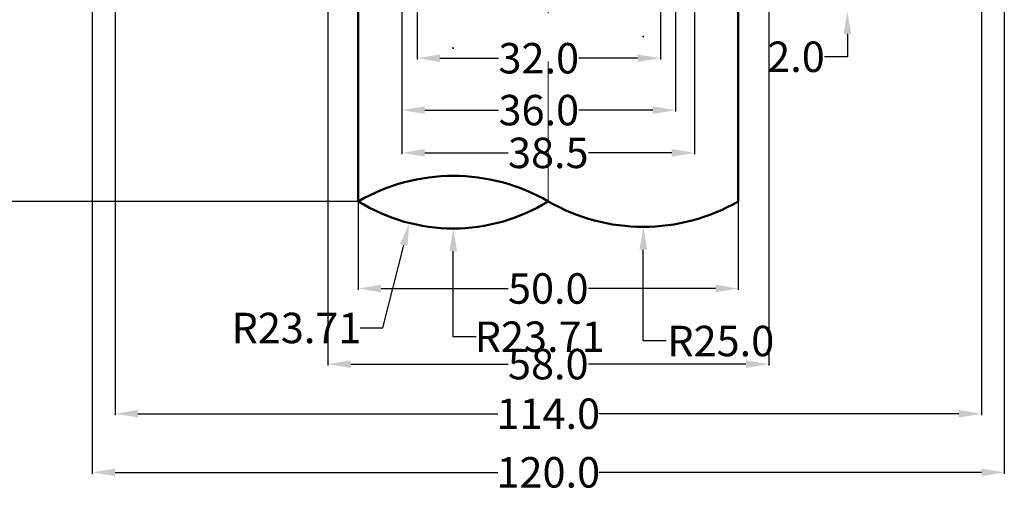
# Model space of a CAD drawing. Units: millimetres. Extents: x 285 to 514, y 588 to 771.
# Tile 2 of 3: x 363 to 492, y 588 to 650. Entities that reach past the tile are written whole.
import ezdxf

# ---------------------------------------------------------------- set-up
doc = ezdxf.new("R2010")
doc.units = ezdxf.units.MM
doc.header["$MEASUREMENT"] = 0
doc.linetypes.add('CENTER', pattern=[50.8, 31.75, -6.35, 6.35, -6.35])
for name, color, linetype, lineweight in [('M-CNTR', 1, 'CENTER', 18), ('M-DIMS', 2, 'Continuous', 25), ('M-OUTL', 7, 'Continuous', 50)]:
    doc.layers.add(name, color=color, linetype=linetype, lineweight=lineweight)
doc.styles.get("Standard").update_dxf_attribs({"font": 'arial.ttf'})
doc.dimstyles.get("Standard").update_dxf_attribs({"dimtxt": 4, "dimasz": 3, "dimexe": 0.18, "dimexo": 0.0625, "dimgap": 0.09, "dimtad": 0, "dimtoh": 1, "dimdec": 1, "dimzin": 0, "dimdsep": 46, "dimtxsty": 'Standard', "dimcen": 0.09, "dimadec": 0, "dimazin": 0, "dimtfac": 1, "dimtdec": 1, "dimtofl": 0, "dimtmove": 0, "dimatfit": 3, "dimfxl": 1, "dimtolj": 1, "dimtzin": 0, "dimarcsym": 0})

# ---------------------------------------------------------------- blocks, each defined once
blk = doc.blocks.new('*D1')
at = {"layer": 'Defpoints', "color": 0, "transparency": 16777216}
for p in [(413.04, 651.15), (451.54, 651.15), (451.54, 632.52)]:
    blk.add_point(p, dxfattribs=at)
at = {"layer": 'M-DIMS', "color": 0, "lineweight": -2, "transparency": 16777216}
for p, q in [((413.04, 651.09), (413.04, 632.34)), ((451.54, 651.09), (451.54, 632.34)), ((416.04, 632.52), (426.99, 632.52)), ((448.54, 632.52), (437.59, 632.52))]:
    blk.add_line(p, q, dxfattribs=at)
at = {"layer": 'M-DIMS', "color": 0, "transparency": 16777216}
for points in [[(416.04, 633.02), (416.04, 632.02), (413.04, 632.52)], [(448.54, 633.02), (448.54, 632.02), (451.54, 632.52)]]:
    blk.add_solid(points, dxfattribs=at)
at = {"layer": 'M-DIMS', "color": 0, "transparency": 16777216, "insert": (432.29, 632.52), "char_height": 4, "attachment_point": 5}
blk.add_mtext('\\A1;38.5', dxfattribs=at)
blk = doc.blocks.new('*D2')
at = {"layer": 'Defpoints', "color": 0, "transparency": 16777216}
for p in [(449.04, 656.31), (413.04, 648.81), (449.04, 638.14)]:
    blk.add_point(p, dxfattribs=at)
at = {"layer": 'M-DIMS', "color": 0, "lineweight": -2, "transparency": 16777216}
for p, q in [((449.04, 656.25), (449.04, 637.96)), ((413.04, 648.75), (413.04, 637.96)), ((416.04, 638.14), (425.76, 638.14)), ((446.04, 638.14), (436.31, 638.14))]:
    blk.add_line(p, q, dxfattribs=at)
at = {"layer": 'M-DIMS', "color": 0, "transparency": 16777216}
for points in [[(416.04, 638.64), (416.04, 637.64), (413.04, 638.14)], [(446.04, 638.64), (446.04, 637.64), (449.04, 638.14)]]:
    blk.add_solid(points, dxfattribs=at)
at = {"layer": 'M-DIMS', "color": 0, "transparency": 16777216, "insert": (431.04, 638.14), "char_height": 4, "attachment_point": 5}
blk.add_mtext('\\A1;36.0', dxfattribs=at)
blk = doc.blocks.new('*D4')
at = {"layer": 'Defpoints', "color": 0, "transparency": 16777216}
for p in [(372.29, 651.15), (492.29, 651.15), (492.29, 590.54)]:
    blk.add_point(p, dxfattribs=at)
at = {"layer": 'M-DIMS', "color": 0, "lineweight": -2, "transparency": 16777216}
for p, q in [((372.29, 651.09), (372.29, 590.36)), ((492.29, 651.09), (492.29, 590.36)), ((375.29, 590.54), (425.64, 590.54)), ((489.29, 590.54), (438.93, 590.54))]:
    blk.add_line(p, q, dxfattribs=at)
at = {"layer": 'M-DIMS', "color": 0, "transparency": 16777216}
for points in [[(375.29, 591.04), (375.29, 590.04), (372.29, 590.54)], [(489.29, 591.04), (489.29, 590.04), (492.29, 590.54)]]:
    blk.add_solid(points, dxfattribs=at)
at = {"layer": 'M-DIMS', "color": 0, "transparency": 16777216, "insert": (432.29, 590.54), "char_height": 4, "attachment_point": 5}
blk.add_mtext('\\A1;120.0', dxfattribs=at)
blk = doc.blocks.new('*D5')
at = {"layer": 'Defpoints', "color": 0, "transparency": 16777216}
for p in [(375.29, 651.15), (489.29, 651.15), (489.29, 598.24)]:
    blk.add_point(p, dxfattribs=at)
at = {"layer": 'M-DIMS', "color": 0, "lineweight": -2, "transparency": 16777216}
for p, q in [((375.29, 651.09), (375.29, 598.06)), ((489.29, 651.09), (489.29, 598.06)), ((378.29, 598.24), (425.64, 598.24)), ((486.29, 598.24), (438.93, 598.24))]:
    blk.add_line(p, q, dxfattribs=at)
at = {"layer": 'M-DIMS', "color": 0, "transparency": 16777216}
for points in [[(378.29, 598.74), (378.29, 597.74), (375.29, 598.24)], [(486.29, 598.74), (486.29, 597.74), (489.29, 598.24)]]:
    blk.add_solid(points, dxfattribs=at)
at = {"layer": 'M-DIMS', "color": 0, "transparency": 16777216, "insert": (432.29, 598.24), "char_height": 4, "attachment_point": 5}
blk.add_mtext('\\A1;114.0', dxfattribs=at)
blk = doc.blocks.new('*D6')
at = {"layer": 'Defpoints', "color": 0, "transparency": 16777216}
for p in [(403.29, 651.15), (461.29, 651.15), (461.29, 604.76)]:
    blk.add_point(p, dxfattribs=at)
at = {"layer": 'M-DIMS', "color": 0, "lineweight": -2, "transparency": 16777216}
for p, q in [((403.29, 651.09), (403.29, 604.58)), ((461.29, 651.09), (461.29, 604.58)), ((406.29, 604.76), (427.01, 604.76)), ((458.29, 604.76), (437.57, 604.76))]:
    blk.add_line(p, q, dxfattribs=at)
at = {"layer": 'M-DIMS', "color": 0, "transparency": 16777216}
for points in [[(406.29, 605.26), (406.29, 604.26), (403.29, 604.76)], [(458.29, 605.26), (458.29, 604.26), (461.29, 604.76)]]:
    blk.add_solid(points, dxfattribs=at)
at = {"layer": 'M-DIMS', "color": 0, "transparency": 16777216, "insert": (432.29, 604.76), "char_height": 4, "attachment_point": 5}
blk.add_mtext('\\A1;58.0', dxfattribs=at)
blk = doc.blocks.new('*D7')
at = {"layer": 'Defpoints', "color": 0, "transparency": 16777216}
for p in [(407.29, 626.15), (457.29, 626.15), (457.29, 614.7)]:
    blk.add_point(p, dxfattribs=at)
at = {"layer": 'M-DIMS', "color": 0, "lineweight": -2, "transparency": 16777216}
for p, q in [((407.29, 626.09), (407.29, 614.52)), ((457.29, 626.09), (457.29, 614.52)), ((410.29, 614.7), (427.01, 614.7)), ((454.29, 614.7), (437.57, 614.7))]:
    blk.add_line(p, q, dxfattribs=at)
at = {"layer": 'M-DIMS', "color": 0, "transparency": 16777216}
for points in [[(410.29, 615.2), (410.29, 614.2), (407.29, 614.7)], [(454.29, 615.2), (454.29, 614.2), (457.29, 614.7)]]:
    blk.add_solid(points, dxfattribs=at)
at = {"layer": 'M-DIMS', "color": 0, "transparency": 16777216, "insert": (432.29, 614.7), "char_height": 4, "attachment_point": 5}
blk.add_mtext('\\A1;50.0', dxfattribs=at)
blk = doc.blocks.new('*D8')
at = {"layer": 'Defpoints', "color": 0, "transparency": 16777216}
for p in [(415.04, 651.15), (447.04, 651.15), (447.04, 644.96)]:
    blk.add_point(p, dxfattribs=at)
at = {"layer": 'M-DIMS', "color": 0, "lineweight": -2, "transparency": 16777216}
for p, q in [((415.04, 651.09), (415.04, 644.78)), ((447.04, 651.09), (447.04, 644.78)), ((418.04, 644.96), (425.76, 644.96)), ((444.04, 644.96), (436.31, 644.96))]:
    blk.add_line(p, q, dxfattribs=at)
at = {"layer": 'M-DIMS', "color": 0, "transparency": 16777216}
for points in [[(418.04, 645.46), (418.04, 644.46), (415.04, 644.96)], [(444.04, 645.46), (444.04, 644.46), (447.04, 644.96)]]:
    blk.add_solid(points, dxfattribs=at)
at = {"layer": 'M-DIMS', "color": 0, "transparency": 16777216, "insert": (431.04, 644.96), "char_height": 4, "attachment_point": 5}
blk.add_mtext('\\A1;32.0', dxfattribs=at)
blk = doc.blocks.new('*D19')
at = {"layer": 'Defpoints', "color": 0, "transparency": 16777216}
for p in [(449.04, 653.15), (449.04, 651.15), (471.64, 651.15)]:
    blk.add_point(p, dxfattribs=at)
at = {"layer": 'M-DIMS', "color": 0, "lineweight": -2, "transparency": 16777216}
for p, q in [((471.64, 656.15), (471.64, 659.15)), ((449.1, 653.15), (471.82, 653.15)), ((449.1, 651.15), (471.82, 651.15)), ((471.64, 648.15), (471.64, 645.15)), ((471.64, 645.15), (468.64, 645.15))]:
    blk.add_line(p, q, dxfattribs=at)
at = {"layer": 'M-DIMS', "color": 0, "transparency": 16777216}
for points in [[(471.14, 656.15), (472.14, 656.15), (471.64, 653.15)], [(471.14, 648.15), (472.14, 648.15), (471.64, 651.15)]]:
    blk.add_solid(points, dxfattribs=at)
at = {"layer": 'M-DIMS', "color": 0, "transparency": 16777216, "insert": (464.88, 645.15), "char_height": 4, "attachment_point": 5}
blk.add_mtext('\\A1;2.0', dxfattribs=at)
blk = doc.blocks.new('*D23')
at = {"layer": 'Defpoints', "color": 0, "transparency": 16777216}
for p in [(407.29, 651.15), (354.44, 626.15), (407.29, 626.15)]:
    blk.add_point(p, dxfattribs=at)
at = {"layer": 'M-DIMS', "color": 0, "lineweight": -2, "transparency": 16777216}
for p, q in [((407.22, 651.15), (354.26, 651.15)), ((354.44, 648.15), (354.44, 643.96)), ((354.44, 629.15), (354.44, 633.34)), ((407.22, 626.15), (354.26, 626.15))]:
    blk.add_line(p, q, dxfattribs=at)
at = {"layer": 'M-DIMS', "color": 0, "transparency": 16777216}
for points in [[(353.94, 648.15), (354.94, 648.15), (354.44, 651.15)], [(353.94, 629.15), (354.94, 629.15), (354.44, 626.15)]]:
    blk.add_solid(points, dxfattribs=at)
at = {"layer": 'M-DIMS', "color": 0, "transparency": 16777216, "insert": (354.44, 638.65), "char_height": 4, "attachment_point": 5, "rotation": 90}
blk.add_mtext('\\A1;25.0', dxfattribs=at)
blk = doc.blocks.new('*D28')
at = {"layer": 'Defpoints', "color": 0, "transparency": 16777216}
for p in [(419.79, 646.3), (419.79, 622.59)]:
    blk.add_point(p, dxfattribs=at)
at = {"layer": 'M-DIMS', "color": 0, "lineweight": -2, "transparency": 16777216}
for p, q in [((419.7, 646.3), (419.88, 646.3)), ((419.79, 646.21), (419.79, 646.39)), ((419.79, 608.36), (419.79, 619.59)), ((422.79, 608.36), (419.79, 608.36))]:
    blk.add_line(p, q, dxfattribs=at)
at = {"layer": 'M-DIMS', "color": 0, "transparency": 16777216}
blk.add_solid([(420.29, 619.59), (419.29, 619.59), (419.79, 622.59)], dxfattribs=at)
at = {"layer": 'M-DIMS', "color": 0, "transparency": 16777216, "insert": (431.15, 608.36), "char_height": 4, "attachment_point": 5}
blk.add_mtext('\\A1;R23.71', dxfattribs=at)
blk = doc.blocks.new('*D29')
at = {"layer": 'Defpoints', "color": 0, "transparency": 16777216}
for p in [(444.79, 647.8), (444.79, 622.8)]:
    blk.add_point(p, dxfattribs=at)
at = {"layer": 'M-DIMS', "color": 0, "lineweight": -2, "transparency": 16777216}
for p, q in [((444.7, 647.8), (444.88, 647.8)), ((444.79, 647.71), (444.79, 647.89)), ((444.79, 607.8), (444.79, 619.8)), ((447.79, 607.8), (444.79, 607.8))]:
    blk.add_line(p, q, dxfattribs=at)
at = {"layer": 'M-DIMS', "color": 0, "transparency": 16777216}
blk.add_solid([(445.29, 619.8), (444.29, 619.8), (444.79, 622.8)], dxfattribs=at)
at = {"layer": 'M-DIMS', "color": 0, "transparency": 16777216, "insert": (454.98, 607.8), "char_height": 4, "attachment_point": 5}
blk.add_mtext('\\A1;R25.0', dxfattribs=at)
blk = doc.blocks.new('*D34')
at = {"layer": 'Defpoints', "color": 0, "transparency": 16777216}
for p in [(419.79, 646.3), (414, 623.3)]:
    blk.add_point(p, dxfattribs=at)
at = {"layer": 'M-DIMS', "color": 0, "lineweight": -2, "transparency": 16777216}
for p, q in [((419.7, 646.3), (419.88, 646.3)), ((419.79, 646.21), (419.79, 646.39)), ((410.53, 609.51), (413.27, 620.39)), ((407.53, 609.51), (410.53, 609.51))]:
    blk.add_line(p, q, dxfattribs=at)
at = {"layer": 'M-DIMS', "color": 0, "transparency": 16777216}
blk.add_solid([(412.78, 620.52), (413.75, 620.27), (414, 623.3)], dxfattribs=at)
at = {"layer": 'M-DIMS', "color": 0, "transparency": 16777216, "insert": (399.16, 609.51), "char_height": 4, "attachment_point": 5}
blk.add_mtext('\\A1;R23.71', dxfattribs=at)

msp = doc.modelspace()

# ---------------------------------------------------------------- linework, layer by layer
at = {"layer": 'M-CNTR'}
msp.add_line((432.2869, 746.1492), (432.2869, 626.1492), dxfattribs=at)
at = {"layer": 'M-OUTL'}
for p, q in [((407.2869, 651.1492), (407.2869, 626.1492)), ((457.2869, 651.1492), (457.2869, 626.1492))]:
    msp.add_line(p, q, dxfattribs=at)
for centre, radius, start, end in [((419.7869, 604.4986), 25, 60, 120), ((419.7869, 646.2978), 23.7111, 238.184885, 301.815115), ((444.7869, 647.7999), 25, 240, 300)]:
    msp.add_arc(centre, radius, start, end, dxfattribs=at)

# ---------------------------------------------------------------- dimensions: what is measured, and where the dimension line sits
at = {"layer": 'M-DIMS'}
for base, p1, p2, override, picture, middle in [((471.6369, 651.1492), (449.0369, 653.1492), (449.0369, 651.1492), {"dimclrd": 0, "dimclre": 0, "dimclrt": 0}, '*D19', (464.8784, 645.1492)), ((354.4384, 626.1492), (407.2869, 651.1492), (407.2869, 626.1492), {"dimdec": 1, "dimlfac": 1, "dimrnd": 0, "dimzin": 0, "dimdsep": 46, "dimlunit": 2}, '*D23', (354.4384, 638.6492))]:
    dim = msp.add_linear_dim(base=base, p1=p1, p2=p2, angle=90, dimstyle='Standard', override=override, dxfattribs=at)
    dim.commit()
    dim.dimension.update_dxf_attribs({"geometry": picture, "text_midpoint": middle})
for base, p1, p2, picture, middle in [((449.0369, 638.1418), (413.0369, 648.8081), (449.0369, 656.3097), '*D2', (431.0369, 638.1418)), ((492.2869, 590.544), (372.2869, 651.1492), (492.2869, 651.1492), '*D4', (432.2869, 590.544)), ((489.2869, 598.2359), (375.2869, 651.1492), (489.2869, 651.1492), '*D5', (432.2869, 598.2359)), ((461.2869, 604.7571), (403.2869, 651.1492), (461.2869, 651.1492), '*D6', (432.2869, 604.7571)), ((451.5369, 632.5157), (413.0369, 651.1492), (451.5369, 651.1492), '*D1', (432.2869, 632.5157)), ((447.0369, 644.9636), (415.0369, 651.1492), (447.0369, 651.1492), '*D8', (431.0369, 644.9636)), ((457.2869, 614.6988), (407.2869, 626.1492), (457.2869, 626.1492), '*D7', (432.2869, 614.6988))]:
    dim = msp.add_linear_dim(base=base, p1=p1, p2=p2, dimstyle='Standard', override={"dimclrd": 0, "dimclre": 0, "dimclrt": 0}, dxfattribs=at)
    dim.commit()
    dim.dimension.update_dxf_attribs({"geometry": picture, "text_midpoint": middle})
for center, mpoint, override, picture, middle in [((444.7869, 647.7999), (444.787, 622.7999), {"dimdec": 1, "dimlfac": 1, "dimrnd": 0, "dimzin": 0, "dimdsep": 46, "dimlunit": 2}, '*D29', (454.9794, 607.7999)), ((419.7869, 646.2978), (414.0009, 623.3035), {"dimdec": 2, "dimlfac": 1, "dimrnd": 0, "dimzin": 0, "dimdsep": 46, "dimlunit": 2}, '*D34', (399.1623, 609.507)), ((419.7869, 646.2978), (419.787, 622.5867), {"dimdec": 2, "dimlfac": 1, "dimrnd": 0, "dimzin": 0, "dimdsep": 46, "dimlunit": 2}, '*D28', (431.154, 608.3601))]:
    dim = msp.add_radius_dim(center=center, mpoint=mpoint, dimstyle='Standard', override=override, dxfattribs=at)
    dim.commit()
    dim.dimension.update_dxf_attribs({"geometry": picture, "text_midpoint": middle, "dimtype": 164})

doc.saveas('drawing.dxf')
